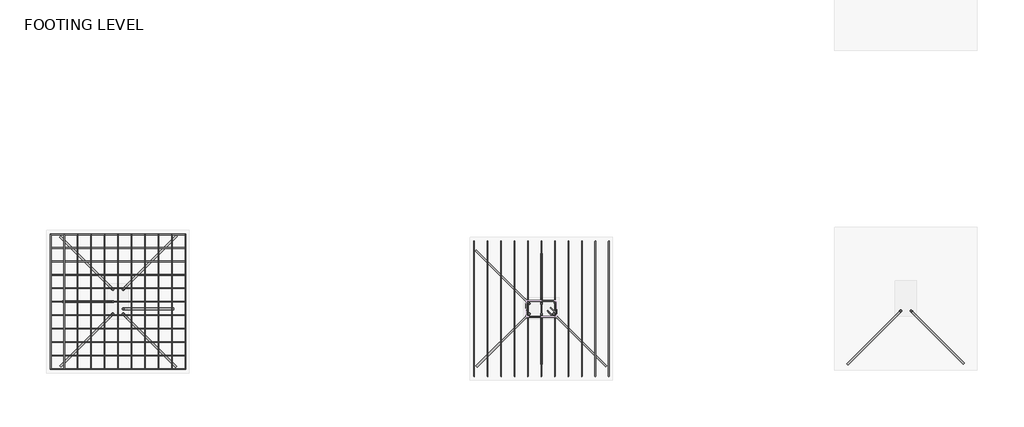
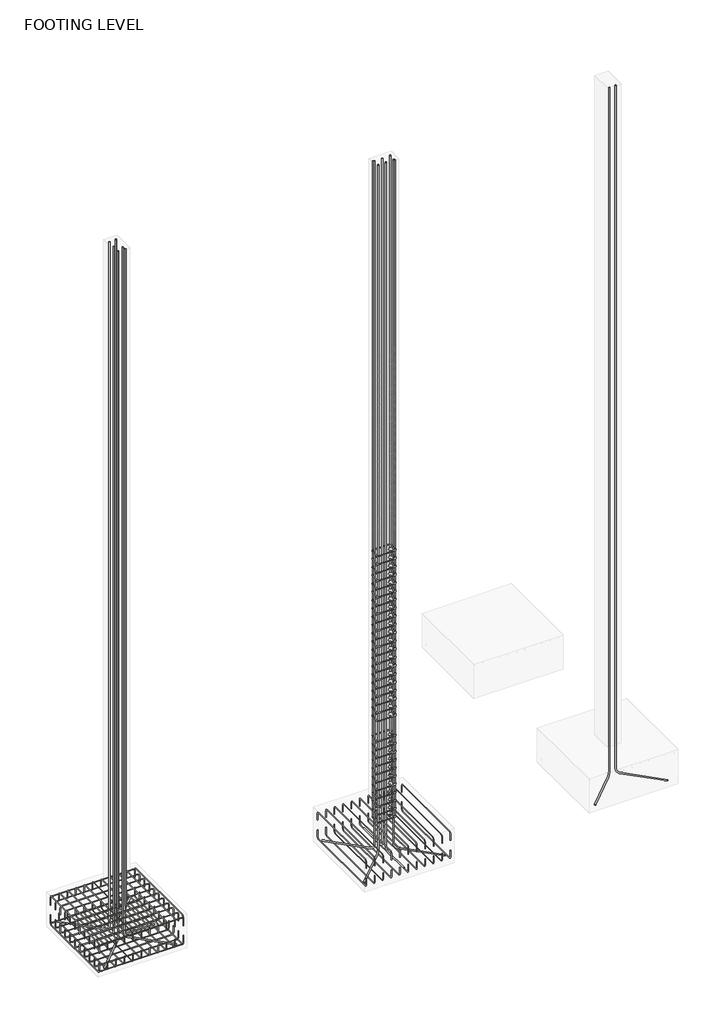
# One storey, part 2 of 10: 27 reinforcing bars.
"""IFC4 building model written with IfcOpenShell, lengths in millimetres."""

from ifc_helpers import new_model, si_unit, point, frame, origin, place, context, project, spatial, polyline, circle_curve, trimmed, segment, composite_curve, source, transform, mapped, element, save
from ifc_brep_helpers import swept_disk

model = new_model("IFC4")

# Units and contexts
model_context = context("Model", 3, world=origin())
ifc_project = project(units=[si_unit("LENGTHUNIT", "METRE", prefix="MILLI")], contexts=[model_context])

# Site, building, storey
site = spatial("IfcSite", under=ifc_project)
building = spatial("IfcBuilding", under=site)
storey = spatial("IfcBuildingStorey", under=building, Name="FOOTING LEVEL", Elevation=-1371.6)

# Reinforcing bars
placement = place(None, origin())
reinforcing_bar_shape = source(origin(), model_context, "Body", "SolidModel", [
    swept_disk(composite_curve([segment(polyline([(-9478.6043223, -565.7798287, -1770.864029), (-9478.6043223, -565.7798287, -1885.164029)]), True, "CONTINUOUS"), segment(trimmed(circle_curve(frame((-9478.6043223, -532.4423287, -1885.164029), z_axis=(1.0, 0.0, 0.0), x_axis=(0.0, -33.33750000000009, 0.0)), 33.3375), [point((-9478.6043223, -565.7798287, -1885.164029))], [point((-9478.6043223, -532.4423287, -1918.501529))], True, "CARTESIAN"), True, "CONTINUOUS"), segment(polyline([(-9478.6043223, -532.4423287, -1918.501529), (-9478.6043223, 839.1576713, -1918.501529)]), True, "CONTINUOUS"), segment(trimmed(circle_curve(frame((-9478.6043223, 839.1576713, -1885.164029), z_axis=(1.0, 0.0, 0.0), x_axis=(0.0, 0.0, -33.337499999999864)), 33.3375), [point((-9478.6043223, 839.1576713, -1918.501529))], [point((-9478.6043223, 872.4951713, -1885.164029))], True, "CARTESIAN"), True, "CONTINUOUS"), segment(polyline([(-9478.6043223, 872.4951713, -1885.164029), (-9478.6043223, 872.4951713, -1770.864029)]), True, "CONTINUOUS")], self_intersect=False), 4.7625),
])
element("IfcReinforcingBar", 1, at=placement, inside=storey, context=model_context, shape_type="MappedRepresentation", body=[
    mapped(reinforcing_bar_shape, transform((0.0, 0.0, 0.0), x_axis=(1.0, 0.0, 0.0), y_axis=(0.0, 1.0, 0.0), z_axis=(0.0, 0.0, 1.0))),
    mapped(reinforcing_bar_shape, transform((-143.8275, 0.0, 0.0), x_axis=(1.0, 0.0, 0.0), y_axis=(0.0, 1.0, 0.0), z_axis=(0.0, 0.0, 1.0))),
    mapped(reinforcing_bar_shape, transform((-287.655, 0.0, 0.0), x_axis=(1.0, 0.0, 0.0), y_axis=(0.0, 1.0, 0.0), z_axis=(0.0, 0.0, 1.0))),
    mapped(reinforcing_bar_shape, transform((-431.4825, 0.0, 0.0), x_axis=(1.0, 0.0, 0.0), y_axis=(0.0, 1.0, 0.0), z_axis=(0.0, 0.0, 1.0))),
    mapped(reinforcing_bar_shape, transform((-575.31, 0.0, 0.0), x_axis=(1.0, 0.0, 0.0), y_axis=(0.0, 1.0, 0.0), z_axis=(0.0, 0.0, 1.0))),
    mapped(reinforcing_bar_shape, transform((-719.1375, 0.0, 0.0), x_axis=(1.0, 0.0, 0.0), y_axis=(0.0, 1.0, 0.0), z_axis=(0.0, 0.0, 1.0))),
    mapped(reinforcing_bar_shape, transform((-862.965, 0.0, 0.0), x_axis=(1.0, 0.0, 0.0), y_axis=(0.0, 1.0, 0.0), z_axis=(0.0, 0.0, 1.0))),
    mapped(reinforcing_bar_shape, transform((-1006.7925, 0.0, 0.0), x_axis=(1.0, 0.0, 0.0), y_axis=(0.0, 1.0, 0.0), z_axis=(0.0, 0.0, 1.0))),
    mapped(reinforcing_bar_shape, transform((-1150.62, 0.0, 0.0), x_axis=(1.0, 0.0, 0.0), y_axis=(0.0, 1.0, 0.0), z_axis=(0.0, 0.0, 1.0))),
    mapped(reinforcing_bar_shape, transform((-1294.4475, 0.0, 0.0), x_axis=(1.0, 0.0, 0.0), y_axis=(0.0, 1.0, 0.0), z_axis=(0.0, 0.0, 1.0))),
    mapped(reinforcing_bar_shape, transform((-1438.275, 0.0, 0.0), x_axis=(1.0, 0.0, 0.0), y_axis=(0.0, 1.0, 0.0), z_axis=(0.0, 0.0, 1.0))),
])
reinforcing_bar_2_shape = source(origin(), model_context, "Body", "SolidModel", [
    swept_disk(composite_curve([segment(polyline([(-10916.8793223, -565.7798287, -1586.5406765), (-10916.8793223, -565.7798287, -1472.2406765)]), True, "CONTINUOUS"), segment(trimmed(circle_curve(frame((-10916.8793223, -532.4423287, -1472.2406765), z_axis=(-1.0, 0.0, 0.0), x_axis=(0.0, -33.33750000000009, 0.0)), 33.3375), [point((-10916.8793223, -565.7798287, -1472.2406765))], [point((-10916.8793223, -532.4423287, -1438.9031765))], True, "CARTESIAN"), True, "CONTINUOUS"), segment(polyline([(-10916.8793223, -532.4423287, -1438.9031765), (-10916.8793223, 839.1576713, -1438.9031765)]), True, "CONTINUOUS"), segment(trimmed(circle_curve(frame((-10916.8793223, 839.1576713, -1472.2406765), z_axis=(-1.0, 0.0, 0.0), x_axis=(0.0, 0.0, 33.33750000000009)), 33.3375), [point((-10916.8793223, 839.1576713, -1438.9031765))], [point((-10916.8793223, 872.4951713, -1472.2406765))], True, "CARTESIAN"), True, "CONTINUOUS"), segment(polyline([(-10916.8793223, 872.4951713, -1472.2406765), (-10916.8793223, 872.4951713, -1586.5406765)]), True, "CONTINUOUS")], self_intersect=False), 4.7625),
])
element("IfcReinforcingBar", 2, at=placement, inside=storey, context=model_context, shape_type="MappedRepresentation", body=[
    mapped(reinforcing_bar_2_shape, transform((0.0, 0.0, 0.0), x_axis=(1.0, 0.0, 0.0), y_axis=(0.0, 1.0, 0.0), z_axis=(0.0, 0.0, 1.0))),
    mapped(reinforcing_bar_2_shape, transform((143.8275, 0.0, 0.0), x_axis=(1.0, 0.0, 0.0), y_axis=(0.0, 1.0, 0.0), z_axis=(0.0, 0.0, 1.0))),
    mapped(reinforcing_bar_2_shape, transform((287.655, 0.0, 0.0), x_axis=(1.0, 0.0, 0.0), y_axis=(0.0, 1.0, 0.0), z_axis=(0.0, 0.0, 1.0))),
    mapped(reinforcing_bar_2_shape, transform((431.4825, 0.0, 0.0), x_axis=(1.0, 0.0, 0.0), y_axis=(0.0, 1.0, 0.0), z_axis=(0.0, 0.0, 1.0))),
    mapped(reinforcing_bar_2_shape, transform((575.31, 0.0, 0.0), x_axis=(1.0, 0.0, 0.0), y_axis=(0.0, 1.0, 0.0), z_axis=(0.0, 0.0, 1.0))),
    mapped(reinforcing_bar_2_shape, transform((719.1375, 0.0, 0.0), x_axis=(1.0, 0.0, 0.0), y_axis=(0.0, 1.0, 0.0), z_axis=(0.0, 0.0, 1.0))),
    mapped(reinforcing_bar_2_shape, transform((862.965, 0.0, 0.0), x_axis=(1.0, 0.0, 0.0), y_axis=(0.0, 1.0, 0.0), z_axis=(0.0, 0.0, 1.0))),
    mapped(reinforcing_bar_2_shape, transform((1006.7925, 0.0, 0.0), x_axis=(1.0, 0.0, 0.0), y_axis=(0.0, 1.0, 0.0), z_axis=(0.0, 0.0, 1.0))),
    mapped(reinforcing_bar_2_shape, transform((1150.62, 0.0, 0.0), x_axis=(1.0, 0.0, 0.0), y_axis=(0.0, 1.0, 0.0), z_axis=(0.0, 0.0, 1.0))),
    mapped(reinforcing_bar_2_shape, transform((1294.4475, 0.0, 0.0), x_axis=(1.0, 0.0, 0.0), y_axis=(0.0, 1.0, 0.0), z_axis=(0.0, 0.0, 1.0))),
    mapped(reinforcing_bar_2_shape, transform((1438.275, 0.0, 0.0), x_axis=(1.0, 0.0, 0.0), y_axis=(0.0, 1.0, 0.0), z_axis=(0.0, 0.0, 1.0))),
])
reinforcing_bar_3_shape = source(origin(), model_context, "Body", "SolidModel", [
    swept_disk(composite_curve([segment(polyline([(-13993.4543223, 948.6951713, -1562.1), (-13993.4543223, 948.6951713, -1447.8)]), True, "CONTINUOUS"), segment(trimmed(circle_curve(frame((-13993.4543223, 915.3576713, -1447.8), z_axis=(1.0, 0.0, 0.0), x_axis=(0.0, 33.33749999999998, 0.0)), 33.3375), [point((-13993.4543223, 948.6951713, -1447.8))], [point((-13993.4543223, 915.3576713, -1414.4625))], True, "CARTESIAN"), True, "CONTINUOUS"), segment(polyline([(-13993.4543223, 915.3576713, -1414.4625), (-13993.4543223, -456.2423287, -1414.4625)]), True, "CONTINUOUS"), segment(trimmed(circle_curve(frame((-13993.4543223, -456.2423287, -1447.8), z_axis=(1.0, 0.0, 0.0), x_axis=(0.0, 0.0, 33.337499999999864)), 33.3375), [point((-13993.4543223, -456.2423287, -1414.4625))], [point((-13993.4543223, -489.5798287, -1447.8))], True, "CARTESIAN"), True, "CONTINUOUS"), segment(polyline([(-13993.4543223, -489.5798287, -1447.8), (-13993.4543223, -489.5798287, -1562.1)]), True, "CONTINUOUS")], self_intersect=False), 4.7625),
])
element("IfcReinforcingBar", 3, at=placement, inside=storey, context=model_context, shape_type="MappedRepresentation", body=[
    mapped(reinforcing_bar_3_shape, transform((0.0, 0.0, 0.0), x_axis=(1.0, 0.0, 0.0), y_axis=(0.0, 1.0, 0.0), z_axis=(0.0, 0.0, 1.0))),
    mapped(reinforcing_bar_3_shape, transform((-143.8275, 0.0, 0.0), x_axis=(1.0, 0.0, 0.0), y_axis=(0.0, 1.0, 0.0), z_axis=(0.0, 0.0, 1.0))),
    mapped(reinforcing_bar_3_shape, transform((-287.655, 0.0, 0.0), x_axis=(1.0, 0.0, 0.0), y_axis=(0.0, 1.0, 0.0), z_axis=(0.0, 0.0, 1.0))),
    mapped(reinforcing_bar_3_shape, transform((-431.4825, 0.0, 0.0), x_axis=(1.0, 0.0, 0.0), y_axis=(0.0, 1.0, 0.0), z_axis=(0.0, 0.0, 1.0))),
    mapped(reinforcing_bar_3_shape, transform((-575.31, 0.0, 0.0), x_axis=(1.0, 0.0, 0.0), y_axis=(0.0, 1.0, 0.0), z_axis=(0.0, 0.0, 1.0))),
    mapped(reinforcing_bar_3_shape, transform((-719.1375, 0.0, 0.0), x_axis=(1.0, 0.0, 0.0), y_axis=(0.0, 1.0, 0.0), z_axis=(0.0, 0.0, 1.0))),
    mapped(reinforcing_bar_3_shape, transform((-862.965, 0.0, 0.0), x_axis=(1.0, 0.0, 0.0), y_axis=(0.0, 1.0, 0.0), z_axis=(0.0, 0.0, 1.0))),
    mapped(reinforcing_bar_3_shape, transform((-1006.7925, 0.0, 0.0), x_axis=(1.0, 0.0, 0.0), y_axis=(0.0, 1.0, 0.0), z_axis=(0.0, 0.0, 1.0))),
    mapped(reinforcing_bar_3_shape, transform((-1150.62, 0.0, 0.0), x_axis=(1.0, 0.0, 0.0), y_axis=(0.0, 1.0, 0.0), z_axis=(0.0, 0.0, 1.0))),
    mapped(reinforcing_bar_3_shape, transform((-1294.4475, 0.0, 0.0), x_axis=(1.0, 0.0, 0.0), y_axis=(0.0, 1.0, 0.0), z_axis=(0.0, 0.0, 1.0))),
    mapped(reinforcing_bar_3_shape, transform((-1438.275, 0.0, 0.0), x_axis=(1.0, 0.0, 0.0), y_axis=(0.0, 1.0, 0.0), z_axis=(0.0, 0.0, 1.0))),
])
reinforcing_bar_4_shape = source(origin(), model_context, "Body", "SolidModel", [
    swept_disk(composite_curve([segment(polyline([(-13993.4543223, -489.5798287, -1790.7), (-13993.4543223, -489.5798287, -1905.0)]), True, "CONTINUOUS"), segment(trimmed(circle_curve(frame((-13993.4543223, -456.2423287, -1905.0), z_axis=(1.0, 0.0, 0.0), x_axis=(0.0, -33.337500000000034, 0.0)), 33.3375), [point((-13993.4543223, -489.5798287, -1905.0))], [point((-13993.4543223, -456.2423287, -1938.3375))], True, "CARTESIAN"), True, "CONTINUOUS"), segment(polyline([(-13993.4543223, -456.2423287, -1938.3375), (-13993.4543223, 915.3576713, -1938.3375)]), True, "CONTINUOUS"), segment(trimmed(circle_curve(frame((-13993.4543223, 915.3576713, -1905.0), z_axis=(1.0, 0.0, 0.0), x_axis=(0.0, 0.0, -33.33750000000009)), 33.3375), [point((-13993.4543223, 915.3576713, -1938.3375))], [point((-13993.4543223, 948.6951713, -1905.0))], True, "CARTESIAN"), True, "CONTINUOUS"), segment(polyline([(-13993.4543223, 948.6951713, -1905.0), (-13993.4543223, 948.6951713, -1790.7)]), True, "CONTINUOUS")], self_intersect=False), 4.7625),
])
element("IfcReinforcingBar", 4, at=placement, inside=storey, context=model_context, shape_type="MappedRepresentation", body=[
    mapped(reinforcing_bar_4_shape, transform((0.0, 0.0, 0.0), x_axis=(1.0, 0.0, 0.0), y_axis=(0.0, 1.0, 0.0), z_axis=(0.0, 0.0, 1.0))),
    mapped(reinforcing_bar_4_shape, transform((-143.8275, 0.0, 0.0), x_axis=(1.0, 0.0, 0.0), y_axis=(0.0, 1.0, 0.0), z_axis=(0.0, 0.0, 1.0))),
    mapped(reinforcing_bar_4_shape, transform((-287.655, 0.0, 0.0), x_axis=(1.0, 0.0, 0.0), y_axis=(0.0, 1.0, 0.0), z_axis=(0.0, 0.0, 1.0))),
    mapped(reinforcing_bar_4_shape, transform((-431.4825, 0.0, 0.0), x_axis=(1.0, 0.0, 0.0), y_axis=(0.0, 1.0, 0.0), z_axis=(0.0, 0.0, 1.0))),
    mapped(reinforcing_bar_4_shape, transform((-575.31, 0.0, 0.0), x_axis=(1.0, 0.0, 0.0), y_axis=(0.0, 1.0, 0.0), z_axis=(0.0, 0.0, 1.0))),
    mapped(reinforcing_bar_4_shape, transform((-719.1375, 0.0, 0.0), x_axis=(1.0, 0.0, 0.0), y_axis=(0.0, 1.0, 0.0), z_axis=(0.0, 0.0, 1.0))),
    mapped(reinforcing_bar_4_shape, transform((-862.965, 0.0, 0.0), x_axis=(1.0, 0.0, 0.0), y_axis=(0.0, 1.0, 0.0), z_axis=(0.0, 0.0, 1.0))),
    mapped(reinforcing_bar_4_shape, transform((-1006.7925, 0.0, 0.0), x_axis=(1.0, 0.0, 0.0), y_axis=(0.0, 1.0, 0.0), z_axis=(0.0, 0.0, 1.0))),
    mapped(reinforcing_bar_4_shape, transform((-1150.62, 0.0, 0.0), x_axis=(1.0, 0.0, 0.0), y_axis=(0.0, 1.0, 0.0), z_axis=(0.0, 0.0, 1.0))),
    mapped(reinforcing_bar_4_shape, transform((-1294.4475, 0.0, 0.0), x_axis=(1.0, 0.0, 0.0), y_axis=(0.0, 1.0, 0.0), z_axis=(0.0, 0.0, 1.0))),
    mapped(reinforcing_bar_4_shape, transform((-1438.275, 0.0, 0.0), x_axis=(1.0, 0.0, 0.0), y_axis=(0.0, 1.0, 0.0), z_axis=(0.0, 0.0, 1.0))),
])
reinforcing_bar_5_shape = source(origin(), model_context, "Body", "SolidModel", [
    swept_disk(composite_curve([segment(polyline([(-15431.7293223, -489.5798287, -1770.864029), (-15431.7293223, -489.5798287, -1885.164029)]), True, "CONTINUOUS"), segment(trimmed(circle_curve(frame((-15398.3918223, -489.5798287, -1885.164029), z_axis=(0.0, -1.0, 0.0), x_axis=(-33.337499999999636, 0.0, 0.0)), 33.3375), [point((-15431.7293223, -489.5798287, -1885.164029))], [point((-15398.3918223, -489.5798287, -1918.501529))], True, "CARTESIAN"), True, "CONTINUOUS"), segment(polyline([(-15398.3918223, -489.5798287, -1918.501529), (-14026.7918223, -489.5798287, -1918.501529)]), True, "CONTINUOUS"), segment(trimmed(circle_curve(frame((-14026.7918223, -489.5798287, -1885.164029), z_axis=(0.0, -1.0, 0.0), x_axis=(0.0, 0.0, -33.337499999999864)), 33.3375), [point((-14026.7918223, -489.5798287, -1918.501529))], [point((-13993.4543223, -489.5798287, -1885.164029))], True, "CARTESIAN"), True, "CONTINUOUS"), segment(polyline([(-13993.4543223, -489.5798287, -1885.164029), (-13993.4543223, -489.5798287, -1770.864029)]), True, "CONTINUOUS")], self_intersect=False), 4.7625),
])
element("IfcReinforcingBar", 5, at=placement, inside=storey, context=model_context, shape_type="MappedRepresentation", body=[
    mapped(reinforcing_bar_5_shape, transform((0.0, 0.0, 0.0), x_axis=(1.0, 0.0, 0.0), y_axis=(0.0, 1.0, 0.0), z_axis=(0.0, 0.0, 1.0))),
    mapped(reinforcing_bar_5_shape, transform((0.0, 143.8275, 0.0), x_axis=(1.0, 0.0, 0.0), y_axis=(0.0, 1.0, 0.0), z_axis=(0.0, 0.0, 1.0))),
    mapped(reinforcing_bar_5_shape, transform((0.0, 287.655, 0.0), x_axis=(1.0, 0.0, 0.0), y_axis=(0.0, 1.0, 0.0), z_axis=(0.0, 0.0, 1.0))),
    mapped(reinforcing_bar_5_shape, transform((0.0, 431.4825, 0.0), x_axis=(1.0, 0.0, 0.0), y_axis=(0.0, 1.0, 0.0), z_axis=(0.0, 0.0, 1.0))),
    mapped(reinforcing_bar_5_shape, transform((0.0, 575.31, 0.0), x_axis=(1.0, 0.0, 0.0), y_axis=(0.0, 1.0, 0.0), z_axis=(0.0, 0.0, 1.0))),
    mapped(reinforcing_bar_5_shape, transform((0.0, 719.1375, 0.0), x_axis=(1.0, 0.0, 0.0), y_axis=(0.0, 1.0, 0.0), z_axis=(0.0, 0.0, 1.0))),
    mapped(reinforcing_bar_5_shape, transform((0.0, 862.965, 0.0), x_axis=(1.0, 0.0, 0.0), y_axis=(0.0, 1.0, 0.0), z_axis=(0.0, 0.0, 1.0))),
    mapped(reinforcing_bar_5_shape, transform((0.0, 1006.7925, 0.0), x_axis=(1.0, 0.0, 0.0), y_axis=(0.0, 1.0, 0.0), z_axis=(0.0, 0.0, 1.0))),
    mapped(reinforcing_bar_5_shape, transform((0.0, 1150.62, 0.0), x_axis=(1.0, 0.0, 0.0), y_axis=(0.0, 1.0, 0.0), z_axis=(0.0, 0.0, 1.0))),
    mapped(reinforcing_bar_5_shape, transform((0.0, 1294.4475, 0.0), x_axis=(1.0, 0.0, 0.0), y_axis=(0.0, 1.0, 0.0), z_axis=(0.0, 0.0, 1.0))),
    mapped(reinforcing_bar_5_shape, transform((0.0, 1438.275, 0.0), x_axis=(1.0, 0.0, 0.0), y_axis=(0.0, 1.0, 0.0), z_axis=(0.0, 0.0, 1.0))),
])
reinforcing_bar_6_shape = source(origin(), model_context, "Body", "SolidModel", [
    swept_disk(composite_curve([segment(polyline([(-15431.7293223, 948.6951713, -1586.5406765), (-15431.7293223, 948.6951713, -1472.2406765)]), True, "CONTINUOUS"), segment(trimmed(circle_curve(frame((-15398.3918223, 948.6951713, -1472.2406765), z_axis=(0.0, 1.0, 0.0), x_axis=(-33.337499999999636, 0.0, 0.0)), 33.3375), [point((-15431.7293223, 948.6951713, -1472.2406765))], [point((-15398.3918223, 948.6951713, -1438.9031765))], True, "CARTESIAN"), True, "CONTINUOUS"), segment(polyline([(-15398.3918223, 948.6951713, -1438.9031765), (-14026.7918223, 948.6951713, -1438.9031765)]), True, "CONTINUOUS"), segment(trimmed(circle_curve(frame((-14026.7918223, 948.6951713, -1472.2406765), z_axis=(0.0, 1.0, 0.0), x_axis=(0.0, 0.0, 33.33750000000009)), 33.3375), [point((-14026.7918223, 948.6951713, -1438.9031765))], [point((-13993.4543223, 948.6951713, -1472.2406765))], True, "CARTESIAN"), True, "CONTINUOUS"), segment(polyline([(-13993.4543223, 948.6951713, -1472.2406765), (-13993.4543223, 948.6951713, -1586.5406765)]), True, "CONTINUOUS")], self_intersect=False), 4.7625),
])
element("IfcReinforcingBar", 6, at=placement, inside=storey, context=model_context, shape_type="MappedRepresentation", body=[
    mapped(reinforcing_bar_6_shape, transform((0.0, 0.0, 0.0), x_axis=(1.0, 0.0, 0.0), y_axis=(0.0, 1.0, 0.0), z_axis=(0.0, 0.0, 1.0))),
    mapped(reinforcing_bar_6_shape, transform((0.0, -143.8275, 0.0), x_axis=(1.0, 0.0, 0.0), y_axis=(0.0, 1.0, 0.0), z_axis=(0.0, 0.0, 1.0))),
    mapped(reinforcing_bar_6_shape, transform((0.0, -287.655, 0.0), x_axis=(1.0, 0.0, 0.0), y_axis=(0.0, 1.0, 0.0), z_axis=(0.0, 0.0, 1.0))),
    mapped(reinforcing_bar_6_shape, transform((0.0, -431.4825, 0.0), x_axis=(1.0, 0.0, 0.0), y_axis=(0.0, 1.0, 0.0), z_axis=(0.0, 0.0, 1.0))),
    mapped(reinforcing_bar_6_shape, transform((0.0, -575.31, 0.0), x_axis=(1.0, 0.0, 0.0), y_axis=(0.0, 1.0, 0.0), z_axis=(0.0, 0.0, 1.0))),
    mapped(reinforcing_bar_6_shape, transform((0.0, -719.1375, 0.0), x_axis=(1.0, 0.0, 0.0), y_axis=(0.0, 1.0, 0.0), z_axis=(0.0, 0.0, 1.0))),
    mapped(reinforcing_bar_6_shape, transform((0.0, -862.965, 0.0), x_axis=(1.0, 0.0, 0.0), y_axis=(0.0, 1.0, 0.0), z_axis=(0.0, 0.0, 1.0))),
    mapped(reinforcing_bar_6_shape, transform((0.0, -1006.7925, 0.0), x_axis=(1.0, 0.0, 0.0), y_axis=(0.0, 1.0, 0.0), z_axis=(0.0, 0.0, 1.0))),
    mapped(reinforcing_bar_6_shape, transform((0.0, -1150.62, 0.0), x_axis=(1.0, 0.0, 0.0), y_axis=(0.0, 1.0, 0.0), z_axis=(0.0, 0.0, 1.0))),
    mapped(reinforcing_bar_6_shape, transform((0.0, -1294.4475, 0.0), x_axis=(1.0, 0.0, 0.0), y_axis=(0.0, 1.0, 0.0), z_axis=(0.0, 0.0, 1.0))),
    mapped(reinforcing_bar_6_shape, transform((0.0, -1438.275, 0.0), x_axis=(1.0, 0.0, 0.0), y_axis=(0.0, 1.0, 0.0), z_axis=(0.0, 0.0, 1.0))),
])
reinforcing_bar_7_shape = source(origin(), model_context, "Body", "SolidModel", [
    swept_disk(composite_curve([segment(polyline([(-10134.9189996, 133.0588881, -1341.4375), (-10078.0548026, 76.194691, -1341.4375)]), True, "CONTINUOUS"), segment(trimmed(circle_curve(frame((-10061.2168223, 93.0326713, -1341.4375), z_axis=(0.0, 0.0, 1.0), x_axis=(-16.83798029999889, -16.837980299999998, 0.0)), 23.8125), [point((-10078.0548026, 76.194691, -1341.4375))], [point((-10037.4043223, 93.0326713, -1341.4375))], True, "CARTESIAN"), True, "CONTINUOUS"), segment(polyline([(-10037.4043223, 93.0326713, -1341.4375), (-10037.4043223, 213.6826713, -1341.4375)]), True, "CONTINUOUS"), segment(trimmed(circle_curve(frame((-10061.2168223, 213.6826713, -1341.4375), z_axis=(0.0, 0.0, 1.0), x_axis=(23.8125, 0.0, 0.0)), 23.8125), [point((-10037.4043223, 213.6826713, -1341.4375))], [point((-10061.2168223, 237.4951713, -1341.4375))], True, "CARTESIAN"), True, "CONTINUOUS"), segment(polyline([(-10061.2168223, 237.4951713, -1341.4375), (-10334.2668223, 237.4951713, -1341.4375)]), True, "CONTINUOUS"), segment(trimmed(circle_curve(frame((-10334.2668223, 213.7207273, -1342.7832232), z_axis=(0.0, -0.056513312022655804, 0.9984018457335854), x_axis=(0.0, 23.774444000000017, 1.3457232000000658)), 23.8125), [point((-10334.2668223, 237.4951713, -1341.4375))], [point((-10358.0793223, 213.7207273, -1342.7832232))], True, "CARTESIAN"), True, "CONTINUOUS"), segment(polyline([(-10358.0793223, 213.7207273, -1342.7832232), (-10358.0793223, 92.9946152, -1349.6167768)]), True, "CONTINUOUS"), segment(trimmed(circle_curve(frame((-10334.2668223, 92.9946152, -1349.6167768), z_axis=(0.0, -0.056513312022655804, 0.9984018457335854), x_axis=(-23.8125, 0.0, 0.0)), 23.8125), [point((-10358.0793223, 92.9946152, -1349.6167768))], [point((-10334.2668223, 69.2201713, -1350.9625))], True, "CARTESIAN"), True, "CONTINUOUS"), segment(polyline([(-10334.2668223, 69.2201713, -1350.9625), (-10061.2168223, 69.2201713, -1350.9625)]), True, "CONTINUOUS"), segment(trimmed(circle_curve(frame((-10061.2168223, 93.0326713, -1350.9625), z_axis=(0.0, 0.0, 1.0), x_axis=(0.0, -23.8125, 0.0)), 23.8125), [point((-10061.2168223, 69.2201713, -1350.9625))], [point((-10044.3788421, 109.8706515, -1350.9625))], True, "CARTESIAN"), True, "CONTINUOUS"), segment(polyline([(-10044.3788421, 109.8706515, -1350.9625), (-10101.2430392, 166.7348485, -1350.9625)]), True, "CONTINUOUS")], self_intersect=False), 4.7625),
])
element("IfcReinforcingBar", 7, at=placement, inside=storey, context=model_context, shape_type="MappedRepresentation", body=[
    mapped(reinforcing_bar_7_shape, transform((0.0, 0.0, 0.0), x_axis=(1.0, 0.0, 0.0), y_axis=(0.0, 1.0, 0.0), z_axis=(0.0, 0.0, 1.0))),
    mapped(reinforcing_bar_7_shape, transform((0.0, 0.0, 146.4111662), x_axis=(1.0, 0.0, 0.0), y_axis=(0.0, 1.0, 0.0), z_axis=(0.0, 0.0, 1.0))),
    mapped(reinforcing_bar_7_shape, transform((0.0, 0.0, 292.8223324), x_axis=(1.0, 0.0, 0.0), y_axis=(0.0, 1.0, 0.0), z_axis=(0.0, 0.0, 1.0))),
    mapped(reinforcing_bar_7_shape, transform((0.0, 0.0, 439.2334986), x_axis=(1.0, 0.0, 0.0), y_axis=(0.0, 1.0, 0.0), z_axis=(0.0, 0.0, 1.0))),
    mapped(reinforcing_bar_7_shape, transform((0.0, 0.0, 585.6446648), x_axis=(1.0, 0.0, 0.0), y_axis=(0.0, 1.0, 0.0), z_axis=(0.0, 0.0, 1.0))),
    mapped(reinforcing_bar_7_shape, transform((0.0, 0.0, 732.055831), x_axis=(1.0, 0.0, 0.0), y_axis=(0.0, 1.0, 0.0), z_axis=(0.0, 0.0, 1.0))),
    mapped(reinforcing_bar_7_shape, transform((0.0, 0.0, 878.4669972), x_axis=(1.0, 0.0, 0.0), y_axis=(0.0, 1.0, 0.0), z_axis=(0.0, 0.0, 1.0))),
    mapped(reinforcing_bar_7_shape, transform((0.0, 0.0, 1024.8781634), x_axis=(1.0, 0.0, 0.0), y_axis=(0.0, 1.0, 0.0), z_axis=(0.0, 0.0, 1.0))),
    mapped(reinforcing_bar_7_shape, transform((0.0, 0.0, 1171.2893296), x_axis=(1.0, 0.0, 0.0), y_axis=(0.0, 1.0, 0.0), z_axis=(0.0, 0.0, 1.0))),
    mapped(reinforcing_bar_7_shape, transform((0.0, 0.0, 1317.7004958), x_axis=(1.0, 0.0, 0.0), y_axis=(0.0, 1.0, 0.0), z_axis=(0.0, 0.0, 1.0))),
    mapped(reinforcing_bar_7_shape, transform((0.0, 0.0, 1464.1116619), x_axis=(1.0, 0.0, 0.0), y_axis=(0.0, 1.0, 0.0), z_axis=(0.0, 0.0, 1.0))),
])
element("IfcReinforcingBar", 8, at=placement, inside=storey, context=model_context, shape_type="SolidModel", body=[
    swept_disk(composite_curve([segment(polyline([(-10341.0020144, 220.4178633, -1346.2), (-10341.0020144, 220.4178633, 10490.2)]), True, "CONTINUOUS")], self_intersect=False), 9.525),
])
element("IfcReinforcingBar", 9, at=placement, inside=storey, context=model_context, shape_type="SolidModel", body=[
    swept_disk(composite_curve([segment(polyline([(-10054.4816302, 86.2974792, -1346.2), (-10054.4816302, 86.2974792, 10490.2)]), True, "CONTINUOUS")], self_intersect=False), 9.525),
])
element("IfcReinforcingBar", 10, at=placement, inside=storey, context=model_context, shape_type="SolidModel", body=[
    swept_disk(composite_curve([segment(polyline([(-10054.4816302, 220.4178633, -1346.2), (-10054.4816302, 220.4178633, 10490.2)]), True, "CONTINUOUS")], self_intersect=False), 9.525),
])
element("IfcReinforcingBar", 11, at=placement, inside=storey, context=model_context, shape_type="SolidModel", body=[
    swept_disk(composite_curve([segment(polyline([(-10889.9777703, -462.6782767, -1910.4342608), (-10375.4483591, 51.8511345, -1910.4342608)]), True, "CONTINUOUS"), segment(trimmed(circle_curve(frame((-10375.4483591, 51.8511345, -1843.7592608), z_axis=(0.7071067811865204, -0.7071067811865748, 0.0), x_axis=(0.0, 0.0, -66.67499999999995)), 66.675), [point((-10375.4483591, 51.8511345, -1910.4342608))], [point((-10328.3020144, 98.9974792, -1843.7592608))], True, "CARTESIAN"), True, "CONTINUOUS"), segment(polyline([(-10328.3020144, 98.9974792, -1843.7592608), (-10328.3020144, 98.9974792, 10490.2)]), True, "CONTINUOUS")], self_intersect=False), 9.525),
])
element("IfcReinforcingBar", 12, at=placement, inside=storey, context=model_context, shape_type="SolidModel", body=[
    swept_disk(composite_curve([segment(polyline([(-10897.9961482, 777.4119971, -1910.4342608), (-10375.4483591, 254.864208, -1910.4342608)]), True, "CONTINUOUS"), segment(trimmed(circle_curve(frame((-10375.4483591, 254.864208, -1843.7592608), z_axis=(-0.707106781186525, -0.70710678118657, 0.0), x_axis=(0.0, 0.0, -66.67499999999995)), 66.675), [point((-10375.4483591, 254.864208, -1910.4342608))], [point((-10328.3020144, 207.7178633, -1843.7592608))], True, "CARTESIAN"), True, "CONTINUOUS"), segment(polyline([(-10328.3020144, 207.7178633, -1843.7592608), (-10328.3020144, 207.7178633, 10490.2)]), True, "CONTINUOUS")], self_intersect=False), 9.525),
])
element("IfcReinforcingBar", 13, at=placement, inside=storey, context=model_context, shape_type="SolidModel", body=[
    swept_disk(composite_curve([segment(polyline([(-9508.4625098, -459.7216413, -1910.4342608), (-10020.0352856, 51.8511345, -1910.4342608)]), True, "CONTINUOUS"), segment(trimmed(circle_curve(frame((-10020.0352856, 51.8511345, -1843.7592608), z_axis=(0.7071067811865204, 0.7071067811865748, 0.0), x_axis=(0.0, 0.0, -66.67499999999995)), 66.675), [point((-10020.0352856, 51.8511345, -1910.4342608))], [point((-10067.1816302, 98.9974792, -1843.7592608))], True, "CARTESIAN"), True, "CONTINUOUS"), segment(polyline([(-10067.1816302, 98.9974792, -1843.7592608), (-10067.1816302, 98.9974792, 10490.2)]), True, "CONTINUOUS")], self_intersect=False), 9.525),
])
element("IfcReinforcingBar", 14, at=placement, inside=storey, context=model_context, shape_type="SolidModel", body=[
    swept_disk(composite_curve([segment(polyline([(-10197.7418223, -439.2323973, -1910.4342608), (-10197.7418223, 32.3224792, -1910.4342608)]), True, "CONTINUOUS"), segment(trimmed(circle_curve(frame((-10197.7418223, 32.3224792, -1843.7592608), z_axis=(1.0, 0.0, 0.0), x_axis=(0.0, 0.0, -66.67499999999995)), 66.675), [point((-10197.7418223, 32.3224792, -1910.4342608))], [point((-10197.7418223, 98.9974792, -1843.7592608))], True, "CARTESIAN"), True, "CONTINUOUS"), segment(polyline([(-10197.7418223, 98.9974792, -1843.7592608), (-10197.7418223, 98.9974792, 10490.2)]), True, "CONTINUOUS")], self_intersect=False), 9.525),
])
element("IfcReinforcingBar", 15, at=placement, inside=storey, context=model_context, shape_type="SolidModel", body=[
    swept_disk(composite_curve([segment(polyline([(-10197.7418223, 745.9477398, -1910.4342608), (-10197.7418223, 274.3928633, -1910.4342608)]), True, "CONTINUOUS"), segment(trimmed(circle_curve(frame((-10197.7418223, 274.3928633, -1843.7592608), z_axis=(-1.0, 0.0, 0.0), x_axis=(0.0, 0.0, -66.67499999999995)), 66.675), [point((-10197.7418223, 274.3928633, -1910.4342608))], [point((-10197.7418223, 207.7178633, -1843.7592608))], True, "CARTESIAN"), True, "CONTINUOUS"), segment(polyline([(-10197.7418223, 207.7178633, -1843.7592608), (-10197.7418223, 207.7178633, 10490.2)]), True, "CONTINUOUS")], self_intersect=False), 9.525),
])
element("IfcReinforcingBar", 16, at=placement, inside=storey, context=model_context, shape_type="SolidModel", body=[
    swept_disk(composite_curve([segment(polyline([(-5695.5058743, -430.9280678, -1910.4342608), (-6210.0352856, 83.6013434, -1910.4342608)]), True, "CONTINUOUS"), segment(trimmed(circle_curve(frame((-6210.0352856, 83.6013434, -1843.7592608), z_axis=(0.7071067811865758, 0.7071067811865194, 0.0), x_axis=(0.0, 0.0, -66.67499999999995)), 66.675), [point((-6210.0352856, 83.6013434, -1910.4342608))], [point((-6257.1816302, 130.7476881, -1843.7592608))], True, "CARTESIAN"), True, "CONTINUOUS"), segment(polyline([(-6257.1816302, 130.7476881, -1843.7592608), (-6257.1816302, 130.7476881, 10477.5)]), True, "CONTINUOUS")], self_intersect=False), 9.525),
])
element("IfcReinforcingBar", 17, at=placement, inside=storey, context=model_context, shape_type="SolidModel", body=[
    swept_disk(composite_curve([segment(polyline([(-6935.5961481, -438.9464456, -1910.4342608), (-6413.048359, 83.6013434, -1910.4342608)]), True, "CONTINUOUS"), segment(trimmed(circle_curve(frame((-6413.048359, 83.6013434, -1843.7592608), z_axis=(0.707106781186569, -0.707106781186526, 0.0), x_axis=(0.0, 0.0, -66.67499999999995)), 66.675), [point((-6413.048359, 83.6013434, -1910.4342608))], [point((-6365.9020144, 130.7476881, -1843.7592608))], True, "CARTESIAN"), True, "CONTINUOUS"), segment(polyline([(-6365.9020144, 130.7476881, -1843.7592608), (-6365.9020144, 130.7476881, 10477.5)]), True, "CONTINUOUS")], self_intersect=False), 9.525),
])
element("IfcReinforcingBar", 18, at=placement, inside=storey, context=model_context, shape_type="SolidModel", body=[
    swept_disk(composite_curve([segment(polyline([(-14645.5316302, 372.8178633, -1346.2), (-14645.5316302, 372.8178633, 10490.2)]), True, "CONTINUOUS")], self_intersect=False), 9.525),
])
element("IfcReinforcingBar", 19, at=placement, inside=storey, context=model_context, shape_type="SolidModel", body=[
    swept_disk(composite_curve([segment(polyline([(-14779.6520144, 86.2974792, -1346.2), (-14779.6520144, 86.2974792, 10490.2)]), True, "CONTINUOUS")], self_intersect=False), 9.525),
])
element("IfcReinforcingBar", 20, at=placement, inside=storey, context=model_context, shape_type="SolidModel", body=[
    swept_disk(composite_curve([segment(polyline([(-14645.5316302, 86.2974792, -1346.2), (-14645.5316302, 86.2974792, 10490.2)]), True, "CONTINUOUS")], self_intersect=False), 9.525),
])
element("IfcReinforcingBar", 21, at=placement, inside=storey, context=model_context, shape_type="SolidModel", body=[
    swept_disk(composite_curve([segment(polyline([(-15328.6277703, 921.7936192, -1910.4342608), (-14814.0983591, 407.264208, -1910.4342608)]), True, "CONTINUOUS"), segment(trimmed(circle_curve(frame((-14814.0983591, 407.264208, -1843.7592608), z_axis=(-0.7071067811865736, -0.7071067811865216, 0.0), x_axis=(0.0, 0.0, -66.67499999999995)), 66.675), [point((-14814.0983591, 407.264208, -1910.4342608))], [point((-14766.9520144, 360.1178633, -1843.7592608))], True, "CARTESIAN"), True, "CONTINUOUS"), segment(polyline([(-14766.9520144, 360.1178633, -1843.7592608), (-14766.9520144, 360.1178633, 10490.2)]), True, "CONTINUOUS")], self_intersect=False), 9.525),
])
element("IfcReinforcingBar", 22, at=placement, inside=storey, context=model_context, shape_type="SolidModel", body=[
    swept_disk(composite_curve([segment(polyline([(-14088.5374965, 929.8119971, -1910.4342608), (-14611.0852856, 407.264208, -1910.4342608)]), True, "CONTINUOUS"), segment(trimmed(circle_curve(frame((-14611.0852856, 407.264208, -1843.7592608), z_axis=(-0.7071067811865712, 0.7071067811865238, 0.0), x_axis=(0.0, 0.0, -66.67499999999995)), 66.675), [point((-14611.0852856, 407.264208, -1910.4342608))], [point((-14658.2316302, 360.1178633, -1843.7592608))], True, "CARTESIAN"), True, "CONTINUOUS"), segment(polyline([(-14658.2316302, 360.1178633, -1843.7592608), (-14658.2316302, 360.1178633, 10490.2)]), True, "CONTINUOUS")], self_intersect=False), 9.525),
])
element("IfcReinforcingBar", 23, at=placement, inside=storey, context=model_context, shape_type="SolidModel", body=[
    swept_disk(composite_curve([segment(polyline([(-15325.6711349, -459.7216413, -1910.4342608), (-14814.0983591, 51.8511345, -1910.4342608)]), True, "CONTINUOUS"), segment(trimmed(circle_curve(frame((-14814.0983591, 51.8511345, -1843.7592608), z_axis=(0.707106781186576, -0.7071067811865192, 0.0), x_axis=(0.0, 0.0, -66.67499999999995)), 66.675), [point((-14814.0983591, 51.8511345, -1910.4342608))], [point((-14766.9520144, 98.9974792, -1843.7592608))], True, "CARTESIAN"), True, "CONTINUOUS"), segment(polyline([(-14766.9520144, 98.9974792, -1843.7592608), (-14766.9520144, 98.9974792, 10490.2)]), True, "CONTINUOUS")], self_intersect=False), 9.525),
])
element("IfcReinforcingBar", 24, at=placement, inside=storey, context=model_context, shape_type="SolidModel", body=[
    swept_disk(composite_curve([segment(polyline([(-14094.0528099, -465.1813412, -1910.4342608), (-14611.0852856, 51.8511345, -1910.4342608)]), True, "CONTINUOUS"), segment(trimmed(circle_curve(frame((-14611.0852856, 51.8511345, -1843.7592608), z_axis=(0.7071067811865689, 0.7071067811865261, 0.0), x_axis=(0.0, 0.0, -66.67499999999995)), 66.675), [point((-14611.0852856, 51.8511345, -1910.4342608))], [point((-14658.2316302, 98.9974792, -1843.7592608))], True, "CARTESIAN"), True, "CONTINUOUS"), segment(polyline([(-14658.2316302, 98.9974792, -1843.7592608), (-14658.2316302, 98.9974792, 10490.2)]), True, "CONTINUOUS")], self_intersect=False), 9.525),
])
element("IfcReinforcingBar", 25, at=placement, inside=storey, context=model_context, shape_type="SolidModel", body=[
    swept_disk(composite_curve([segment(polyline([(-15305.1818909, 229.5576713, -1910.4342608), (-14833.6270144, 229.5576713, -1910.4342608)]), True, "CONTINUOUS"), segment(trimmed(circle_curve(frame((-14833.6270144, 229.5576713, -1843.7592608), z_axis=(0.0, -1.0, 0.0), x_axis=(0.0, 0.0, -66.67499999999995)), 66.675), [point((-14833.6270144, 229.5576713, -1910.4342608))], [point((-14766.9520144, 229.5576713, -1843.7592608))], True, "CARTESIAN"), True, "CONTINUOUS"), segment(polyline([(-14766.9520144, 229.5576713, -1843.7592608), (-14766.9520144, 229.5576713, 10490.2)]), True, "CONTINUOUS")], self_intersect=False), 9.525),
])
element("IfcReinforcingBar", 26, at=placement, inside=storey, context=model_context, shape_type="SolidModel", body=[
    swept_disk(composite_curve([segment(polyline([(-14120.0017538, 153.3576713, -1910.4342608), (-14591.5566302, 153.3576713, -1910.4342608)]), True, "CONTINUOUS"), segment(trimmed(circle_curve(frame((-14591.5566302, 153.3576713, -1843.7592608), z_axis=(0.0, 1.0, 0.0), x_axis=(0.0, 0.0, -66.67499999999995)), 66.675), [point((-14591.5566302, 153.3576713, -1910.4342608))], [point((-14658.2316302, 153.3576713, -1843.7592608))], True, "CARTESIAN"), True, "CONTINUOUS"), segment(polyline([(-14658.2316302, 153.3576713, -1843.7592608), (-14658.2316302, 153.3576713, 10490.2)]), True, "CONTINUOUS")], self_intersect=False), 9.525),
])
reinforcing_bar_8_shape = source(origin(), model_context, "Body", "SolidModel", [
    swept_disk(composite_curve([segment(polyline([(-10134.9189996, 133.0588881, 487.3625), (-10078.0548026, 76.194691, 487.3625)]), True, "CONTINUOUS"), segment(trimmed(circle_curve(frame((-10061.2168223, 93.0326713, 487.3625), z_axis=(0.0, 0.0, 1.0), x_axis=(-16.83798029999889, -16.837980299999998, 0.0)), 23.8125), [point((-10078.0548026, 76.194691, 487.3625))], [point((-10037.4043223, 93.0326713, 487.3625))], True, "CARTESIAN"), True, "CONTINUOUS"), segment(polyline([(-10037.4043223, 93.0326713, 487.3625), (-10037.4043223, 213.6826713, 487.3625)]), True, "CONTINUOUS"), segment(trimmed(circle_curve(frame((-10061.2168223, 213.6826713, 487.3625), z_axis=(0.0, 0.0, 1.0), x_axis=(23.8125, 0.0, 0.0)), 23.8125), [point((-10037.4043223, 213.6826713, 487.3625))], [point((-10061.2168223, 237.4951713, 487.3625))], True, "CARTESIAN"), True, "CONTINUOUS"), segment(polyline([(-10061.2168223, 237.4951713, 487.3625), (-10334.2668223, 237.4951713, 487.3625)]), True, "CONTINUOUS"), segment(trimmed(circle_curve(frame((-10334.2668223, 213.7207273, 486.0167768), z_axis=(0.0, -0.056513312022655804, 0.9984018457335854), x_axis=(0.0, 23.774444000000017, 1.345723200000009)), 23.8125), [point((-10334.2668223, 237.4951713, 487.3625))], [point((-10358.0793223, 213.7207273, 486.0167768))], True, "CARTESIAN"), True, "CONTINUOUS"), segment(polyline([(-10358.0793223, 213.7207273, 486.0167768), (-10358.0793223, 92.9946152, 479.1832232)]), True, "CONTINUOUS"), segment(trimmed(circle_curve(frame((-10334.2668223, 92.9946152, 479.1832232), z_axis=(0.0, -0.056513312022655804, 0.9984018457335854), x_axis=(-23.8125, 0.0, 0.0)), 23.8125), [point((-10358.0793223, 92.9946152, 479.1832232))], [point((-10334.2668223, 69.2201713, 477.8375))], True, "CARTESIAN"), True, "CONTINUOUS"), segment(polyline([(-10334.2668223, 69.2201713, 477.8375), (-10061.2168223, 69.2201713, 477.8375)]), True, "CONTINUOUS"), segment(trimmed(circle_curve(frame((-10061.2168223, 93.0326713, 477.8375), z_axis=(0.0, 0.0, 1.0), x_axis=(0.0, -23.8125, 0.0)), 23.8125), [point((-10061.2168223, 69.2201713, 477.8375))], [point((-10044.3788421, 109.8706515, 477.8375))], True, "CARTESIAN"), True, "CONTINUOUS"), segment(polyline([(-10044.3788421, 109.8706515, 477.8375), (-10101.2430392, 166.7348485, 477.8375)]), True, "CONTINUOUS")], self_intersect=False), 4.7625),
])
element("IfcReinforcingBar", 27, at=placement, inside=storey, context=model_context, shape_type="MappedRepresentation", body=[
    mapped(reinforcing_bar_8_shape, transform((0.0, 0.0, 0.0), x_axis=(1.0, 0.0, 0.0), y_axis=(0.0, 1.0, 0.0), z_axis=(0.0, 0.0, 1.0))),
    mapped(reinforcing_bar_8_shape, transform((0.0, 0.0, 148.9295804), x_axis=(1.0, 0.0, 0.0), y_axis=(0.0, 1.0, 0.0), z_axis=(0.0, 0.0, 1.0))),
    mapped(reinforcing_bar_8_shape, transform((0.0, 0.0, 297.8591609), x_axis=(1.0, 0.0, 0.0), y_axis=(0.0, 1.0, 0.0), z_axis=(0.0, 0.0, 1.0))),
    mapped(reinforcing_bar_8_shape, transform((0.0, 0.0, 446.7887413), x_axis=(1.0, 0.0, 0.0), y_axis=(0.0, 1.0, 0.0), z_axis=(0.0, 0.0, 1.0))),
    mapped(reinforcing_bar_8_shape, transform((0.0, 0.0, 595.7183218), x_axis=(1.0, 0.0, 0.0), y_axis=(0.0, 1.0, 0.0), z_axis=(0.0, 0.0, 1.0))),
    mapped(reinforcing_bar_8_shape, transform((0.0, 0.0, 744.6479022), x_axis=(1.0, 0.0, 0.0), y_axis=(0.0, 1.0, 0.0), z_axis=(0.0, 0.0, 1.0))),
    mapped(reinforcing_bar_8_shape, transform((0.0, 0.0, 893.5774826), x_axis=(1.0, 0.0, 0.0), y_axis=(0.0, 1.0, 0.0), z_axis=(0.0, 0.0, 1.0))),
    mapped(reinforcing_bar_8_shape, transform((0.0, 0.0, 1042.5070631), x_axis=(1.0, 0.0, 0.0), y_axis=(0.0, 1.0, 0.0), z_axis=(0.0, 0.0, 1.0))),
    mapped(reinforcing_bar_8_shape, transform((0.0, 0.0, 1191.4366435), x_axis=(1.0, 0.0, 0.0), y_axis=(0.0, 1.0, 0.0), z_axis=(0.0, 0.0, 1.0))),
    mapped(reinforcing_bar_8_shape, transform((0.0, 0.0, 1340.366224), x_axis=(1.0, 0.0, 0.0), y_axis=(0.0, 1.0, 0.0), z_axis=(0.0, 0.0, 1.0))),
    mapped(reinforcing_bar_8_shape, transform((0.0, 0.0, 1489.2958044), x_axis=(1.0, 0.0, 0.0), y_axis=(0.0, 1.0, 0.0), z_axis=(0.0, 0.0, 1.0))),
    mapped(reinforcing_bar_8_shape, transform((0.0, 0.0, 1638.2253848), x_axis=(1.0, 0.0, 0.0), y_axis=(0.0, 1.0, 0.0), z_axis=(0.0, 0.0, 1.0))),
    mapped(reinforcing_bar_8_shape, transform((0.0, 0.0, 1787.1549653), x_axis=(1.0, 0.0, 0.0), y_axis=(0.0, 1.0, 0.0), z_axis=(0.0, 0.0, 1.0))),
    mapped(reinforcing_bar_8_shape, transform((0.0, 0.0, 1936.0845457), x_axis=(1.0, 0.0, 0.0), y_axis=(0.0, 1.0, 0.0), z_axis=(0.0, 0.0, 1.0))),
    mapped(reinforcing_bar_8_shape, transform((0.0, 0.0, 2085.0141261), x_axis=(1.0, 0.0, 0.0), y_axis=(0.0, 1.0, 0.0), z_axis=(0.0, 0.0, 1.0))),
    mapped(reinforcing_bar_8_shape, transform((0.0, 0.0, 2233.9437066), x_axis=(1.0, 0.0, 0.0), y_axis=(0.0, 1.0, 0.0), z_axis=(0.0, 0.0, 1.0))),
    mapped(reinforcing_bar_8_shape, transform((0.0, 0.0, 2382.873287), x_axis=(1.0, 0.0, 0.0), y_axis=(0.0, 1.0, 0.0), z_axis=(0.0, 0.0, 1.0))),
    mapped(reinforcing_bar_8_shape, transform((0.0, 0.0, 2531.8028675), x_axis=(1.0, 0.0, 0.0), y_axis=(0.0, 1.0, 0.0), z_axis=(0.0, 0.0, 1.0))),
    mapped(reinforcing_bar_8_shape, transform((0.0, 0.0, 2680.7324479), x_axis=(1.0, 0.0, 0.0), y_axis=(0.0, 1.0, 0.0), z_axis=(0.0, 0.0, 1.0))),
    mapped(reinforcing_bar_8_shape, transform((0.0, 0.0, 2829.6620283), x_axis=(1.0, 0.0, 0.0), y_axis=(0.0, 1.0, 0.0), z_axis=(0.0, 0.0, 1.0))),
    mapped(reinforcing_bar_8_shape, transform((0.0, 0.0, 2978.5916088), x_axis=(1.0, 0.0, 0.0), y_axis=(0.0, 1.0, 0.0), z_axis=(0.0, 0.0, 1.0))),
])

save(model, "model.ifc")

# Revit data of these elements
# Elements 1, 2, 3, 4, 5, 6, 7, 8, 9, 10, 11, 12, 13, 14, 15, 16, 17, 18, 19, 20, 21, 22, 23, 24, 25, 26, 27 (IfcReinforcingBar)
#   Phase Created = New Construction
